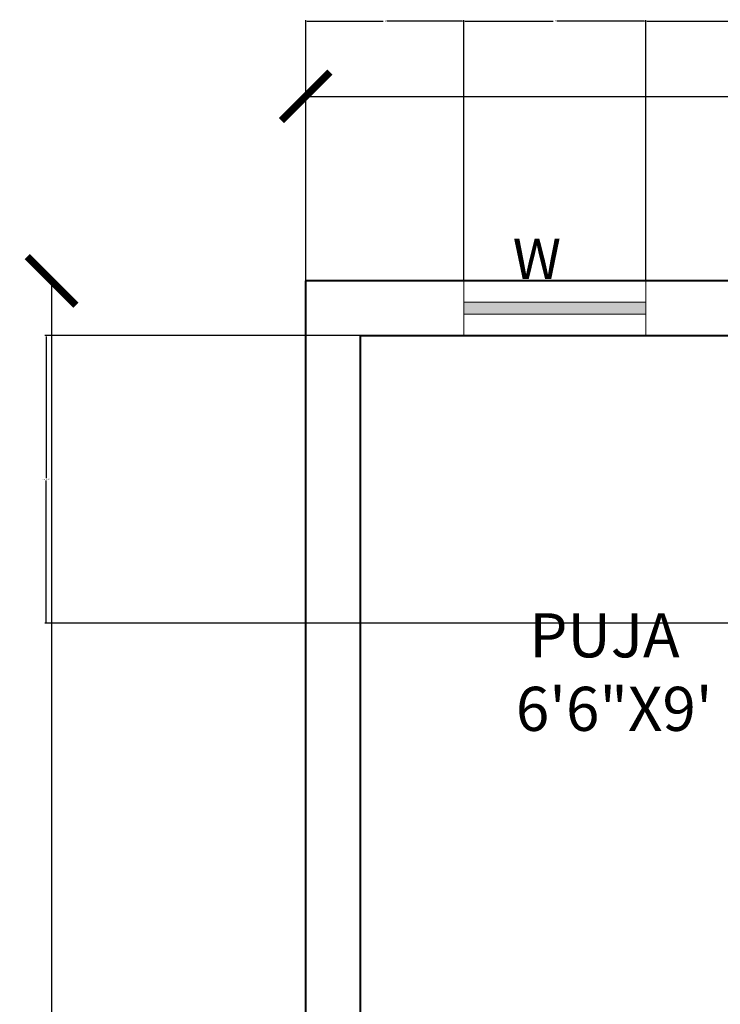
# Model space of a CAD drawing. Units: inches. Extents: x 182 to 1022, y -617 to 111.
# Tile 18 of 33: x 182 to 298, y -120 to 43. Entities that reach past the tile are written whole.
import ezdxf

# ---------------------------------------------------------------- set-up
doc = ezdxf.new("R2010")
doc.units = ezdxf.units.IN
doc.header["$MEASUREMENT"] = 0
for name, color, linetype, lineweight in [('A-ANNO-DIMS', 2, 'Continuous', 18), ('A-ANNO-IDEN', 1, 'Continuous', 18), ('A-AREA-IDEN', 8, 'Continuous', 18), ('A-GLAZ-PATT', 5, 'Continuous', 13), ('wall', 1, 'Continuous', 40), ('wind', 5, 'Continuous', 20)]:
    doc.layers.add(name, color=color, linetype=linetype, lineweight=lineweight)
doc.styles.get("Standard").update_dxf_attribs({"font": 'arial.ttf'})
doc.dimstyles.get("Standard").update_dxf_attribs({"dimtxt": 0.18, "dimasz": 0.18, "dimexe": 0.18, "dimexo": 0.0625, "dimgap": 0.09, "dimtad": 0, "dimtih": 1, "dimtoh": 1, "dimdec": 1, "dimzin": 0, "dimdsep": 46, "dimlunit": 4, "dimtxsty": 'Standard', "dimcen": 0.09, "dimadec": 0, "dimazin": 0, "dimtfac": 1, "dimtdec": 1, "dimtofl": 0, "dimtmove": 0, "dimatfit": 3, "dimfxl": 1, "dimtolj": 1, "dimtzin": 0, "dimarcsym": 0})

# ---------------------------------------------------------------- blocks, each defined once
blk = doc.blocks.new('_ArchTick')
at = {"color": 0, "linetype": 'ByBlock', "const_width": 0.15}
blk.add_lwpolyline([(-0.5, -0.5), (0.5, 0.5)], dxfattribs=at)
blk = doc.blocks.new('*D5')
at = {"layer": 'A-ANNO-DIMS', "color": 0, "lineweight": -2, "transparency": 16777216}
for p, q in [((229.36, 30.06), (387.5, 30.06)), ((565.36, 30.06), (407.22, 30.06))]:
    blk.add_line(p, q, dxfattribs=at)
at = {"layer": 'Defpoints', "color": 0, "transparency": 16777216}
for p in [(565.36, 30.06), (229.36, -0.37), (565.36, -0.37)]:
    blk.add_point(p, dxfattribs=at)
at = {"layer": 'A-ANNO-DIMS', "color": 0, "lineweight": -2, "transparency": 16777216, "xscale": 8, "yscale": 8, "zscale": 8, "rotation": 180}
blk.add_blockref('_ArchTick', (229.36, 30.06), dxfattribs=at)
at = {"layer": 'A-ANNO-DIMS', "color": 0, "lineweight": -2, "transparency": 16777216, "xscale": 8, "yscale": 8, "zscale": 8}
blk.add_blockref('_ArchTick', (565.36, 30.06), dxfattribs=at)
at = {"layer": 'A-ANNO-DIMS', "color": 0, "transparency": 16777216, "insert": (397.36, 30.06), "char_height": 8, "attachment_point": 5}
blk.add_mtext("\\A1;28'", dxfattribs=at)
blk = doc.blocks.new('*D6')
at = {"layer": 'A-ANNO-DIMS', "color": 0, "lineweight": -2, "transparency": 16777216}
for p, q in [((187.47, -0.37), (187.47, -260.42)), ((187.47, -540.37), (187.47, -280.32))]:
    blk.add_line(p, q, dxfattribs=at)
at = {"layer": 'Defpoints', "color": 0, "transparency": 16777216}
for p in [(229.36, -0.37), (187.47, -540.37), (229.36, -540.37)]:
    blk.add_point(p, dxfattribs=at)
at = {"layer": 'A-ANNO-DIMS', "color": 0, "lineweight": -2, "transparency": 16777216, "xscale": 8, "yscale": 8, "zscale": 8}
for p, rotation in [((187.47, -0.37), 90), ((187.47, -540.37), 270)]:
    blk.add_blockref('_ArchTick', p, dxfattribs=dict(at, rotation=rotation))
at = {"layer": 'A-ANNO-DIMS', "color": 0, "transparency": 16777216, "insert": (187.47, -270.37), "char_height": 8, "attachment_point": 5, "rotation": 90}
blk.add_mtext("\\A1;45'", dxfattribs=at)
blk = doc.blocks.new('*D32')
at = {"layer": 'A-ANNO-DIMS', "color": 0, "lineweight": -2, "transparency": 16777216}
for p, q in [((229.36, -0.31), (229.36, 42.61)), ((229.54, 42.43), (242.05, 42.43)), ((255.22, 42.43), (242.71, 42.43)), ((255.4, -0.31), (255.4, 42.61))]:
    blk.add_line(p, q, dxfattribs=at)
at = {"layer": 'A-ANNO-DIMS', "color": 0, "transparency": 16777216}
for points in [[(229.54, 42.46), (229.54, 42.4), (229.36, 42.43)], [(255.22, 42.46), (255.22, 42.4), (255.4, 42.43)]]:
    blk.add_solid(points, dxfattribs=at)
at = {"layer": 'Defpoints', "color": 0, "transparency": 16777216}
for p in [(255.4, 42.43), (229.36, -0.37), (255.4, -0.37)]:
    blk.add_point(p, dxfattribs=at)
at = {"layer": 'A-ANNO-DIMS', "color": 0, "transparency": 16777216, "insert": (242.38, 42.43), "char_height": 0.18, "attachment_point": 5}
blk.add_mtext('\\A1;2\'-2"', dxfattribs=at)
blk = doc.blocks.new('*D33')
at = {"layer": 'A-ANNO-DIMS', "color": 0, "lineweight": -2, "transparency": 16777216}
for p, q in [((255.4, -0.31), (255.4, 42.61)), ((255.58, 42.43), (270.07, 42.43)), ((285.22, 42.43), (270.73, 42.43)), ((285.4, -0.31), (285.4, 42.61))]:
    blk.add_line(p, q, dxfattribs=at)
at = {"layer": 'A-ANNO-DIMS', "color": 0, "transparency": 16777216}
for points in [[(255.58, 42.46), (255.58, 42.4), (255.4, 42.43)], [(285.22, 42.46), (285.22, 42.4), (285.4, 42.43)]]:
    blk.add_solid(points, dxfattribs=at)
at = {"layer": 'Defpoints', "color": 0, "transparency": 16777216}
for p in [(285.4, 42.43), (255.4, -0.37), (285.4, -0.37)]:
    blk.add_point(p, dxfattribs=at)
at = {"layer": 'A-ANNO-DIMS', "color": 0, "transparency": 16777216, "insert": (270.4, 42.43), "char_height": 0.18, "attachment_point": 5}
blk.add_mtext('\\A1;2\'-6"', dxfattribs=at)
blk = doc.blocks.new('*D34')
at = {"layer": 'A-ANNO-DIMS', "color": 0, "lineweight": -2, "transparency": 16777216}
for p, q in [((285.4, -0.31), (285.4, 42.61)), ((285.58, 42.43), (312.2, 42.43)), ((339.91, 42.43), (313.29, 42.43)), ((340.09, -0.31), (340.09, 42.61))]:
    blk.add_line(p, q, dxfattribs=at)
at = {"layer": 'A-ANNO-DIMS', "color": 0, "transparency": 16777216}
for points in [[(285.58, 42.46), (285.58, 42.4), (285.4, 42.43)], [(339.91, 42.46), (339.91, 42.4), (340.09, 42.43)]]:
    blk.add_solid(points, dxfattribs=at)
at = {"layer": 'Defpoints', "color": 0, "transparency": 16777216}
for p in [(340.09, 42.43), (285.4, -0.37), (340.09, -0.37)]:
    blk.add_point(p, dxfattribs=at)
at = {"layer": 'A-ANNO-DIMS', "color": 0, "transparency": 16777216, "insert": (312.75, 42.43), "char_height": 0.18, "attachment_point": 5}
blk.add_mtext('\\A1;4\'-6 1/2"', dxfattribs=at)
blk = doc.blocks.new('*D43')
at = {"layer": 'A-ANNO-DIMS', "color": 0, "lineweight": -2, "transparency": 16777216}
for p, q in [((556.3, -9.37), (186.38, -9.37)), ((186.56, -9.55), (186.56, -32.91)), ((186.56, -56.63), (186.56, -33.28)), ((556.3, -56.81), (186.38, -56.81))]:
    blk.add_line(p, q, dxfattribs=at)
at = {"layer": 'A-ANNO-DIMS', "color": 0, "transparency": 16777216}
for points in [[(186.53, -9.55), (186.59, -9.55), (186.56, -9.37)], [(186.53, -56.63), (186.59, -56.63), (186.56, -56.81)]]:
    blk.add_solid(points, dxfattribs=at)
at = {"layer": 'Defpoints', "color": 0, "transparency": 16777216}
for p in [(556.36, -9.37), (186.56, -56.81), (556.36, -56.81)]:
    blk.add_point(p, dxfattribs=at)
at = {"layer": 'A-ANNO-DIMS', "color": 0, "transparency": 16777216, "insert": (186.56, -33.09), "char_height": 0.18, "attachment_point": 5}
blk.add_mtext('\\A1;3\'-11 1/2"', dxfattribs=at)

msp = doc.modelspace()

# ---------------------------------------------------------------- hatches: boundary and pattern name
at = {"layer": 'A-GLAZ-PATT'}
h = msp.add_hatch(color=256, dxfattribs=at)
h.dxf.hatch_style = 1
h.paths.add_polyline_path([(285.4, -3.87), (255.4, -3.87), (255.4, -5.87), (285.4, -5.87)])
h.paths.add_polyline_path([(376.09, -3.87), (340.09, -3.87), (340.09, -5.87), (376.09, -5.87)])
h.paths.add_polyline_path([(561.86, -132.92), (559.86, -132.92), (559.86, -168.92), (561.86, -168.92)])
h.paths.add_polyline_path([(561.86, -56.81), (559.86, -56.81), (559.86, -86.81), (561.86, -86.81)])
h.paths.add_polyline_path([(561.86, -258.37), (559.86, -258.37), (559.86, -282.37), (561.86, -282.37)])
h.paths.add_polyline_path([(533.36, -534.87), (497.36, -534.87), (497.36, -536.87), (533.36, -536.87)])
h.paths.add_polyline_path([(234.86, -252.37), (232.86, -252.37), (232.86, -288.37), (234.86, -288.37)])

# ---------------------------------------------------------------- linework, layer by layer
at = {"layer": 'wall'}
for p, q in [((229.36, -540.37), (229.36, -0.37)), ((565.36, -0.37), (229.36, -0.37)), ((238.36, -9.37), (238.36, -540.37)), ((238.36, -9.37), (556.36, -9.37))]:
    msp.add_line(p, q, dxfattribs=at)
at = {"layer": 'wind'}
for p, q in [((255.4, -9.37), (255.4, -0.37)), ((285.4, -9.37), (285.4, -0.37)), ((255.4, -3.87), (285.4, -3.87)), ((255.4, -5.87), (285.4, -5.87))]:
    msp.add_line(p, q, dxfattribs=at)

# ---------------------------------------------------------------- texts
at = {"layer": 'A-ANNO-IDEN'}
msp.add_text('W', height=6.65, dxfattribs=at).set_placement((263.48, -0.06))
at = {"layer": 'A-AREA-IDEN', "insert": (264, -55.16), "char_height": 7.2703, "attachment_point": 1}
msp.add_mtext_dynamic_manual_height_columns(' PUJA              6\'6"X9\'', width=33.1677, gutter_width=1.21, heights=[0], dxfattribs=at)

# ---------------------------------------------------------------- dimensions: what is measured, and where the dimension line sits
at = {"layer": 'A-ANNO-DIMS'}
for base, p1, p2, override, picture, middle in [((255.4, 42.43), (229.36, -0.37), (255.4, -0.37), {"dimdec": 1, "dimlfac": 1, "dimrnd": 0, "dimzin": 1, "dimdsep": 46, "dimlunit": 4, "dimfrac": 2}, '*D32', (242.38, 42.43)), ((340.09, 42.43), (285.4, -0.37), (340.09, -0.37), {"dimdec": 1, "dimlfac": 1, "dimrnd": 0, "dimzin": 1, "dimdsep": 46, "dimlunit": 4, "dimfrac": 2}, '*D34', (312.75, 42.43)), ((565.36, 30.06), (229.36, -0.37), (565.36, -0.37), {"dimtxt": 8, "dimasz": 8, "dimgap": 3, "dimblk1": 'ArchTick', "dimblk2": 'ArchTick', "dimsah": 1, "dimse1": 1, "dimse2": 1, "dimsd1": 0, "dimclrd": 0, "dimclre": 0, "dimclrt": 0}, '*D5', (397.36, 30.06))]:
    dim = msp.add_linear_dim(base=base, p1=p1, p2=p2, dimstyle='Standard', override=override, dxfattribs=at)
    dim.commit()
    dim.dimension.update_dxf_attribs({"geometry": picture, "text_midpoint": middle})
for base, p1, p2, angle, override, picture, middle in [((285.4, 42.43), (255.4, -0.37), (285.4, -0.37), 0, {"dimdec": 1, "dimlfac": 1, "dimrnd": 0, "dimzin": 1, "dimdsep": 46, "dimlunit": 4, "dimfrac": 2}, '*D33', (270.4, 42.43)), ((187.47, -540.37), (229.36, -0.37), (229.36, -540.37), 90, {"dimtxt": 8, "dimasz": 8, "dimgap": 3, "dimtih": 0, "dimblk1": 'ArchTick', "dimblk2": 'ArchTick', "dimsah": 1, "dimse1": 1, "dimse2": 1, "dimclrd": 0, "dimclre": 0, "dimclrt": 0}, '*D6', (187.47, -270.37)), ((186.56, -56.81), (556.36, -9.37), (556.36, -56.81), 90, {"dimdec": 1, "dimlfac": 1, "dimrnd": 0, "dimzin": 1, "dimdsep": 46, "dimlunit": 4, "dimfrac": 2}, '*D43', (186.56, -33.09))]:
    dim = msp.add_linear_dim(base=base, p1=p1, p2=p2, angle=angle, dimstyle='Standard', override=override, dxfattribs=at)
    dim.commit()
    dim.dimension.update_dxf_attribs({"geometry": picture, "text_midpoint": middle})

doc.saveas('drawing.dxf')
